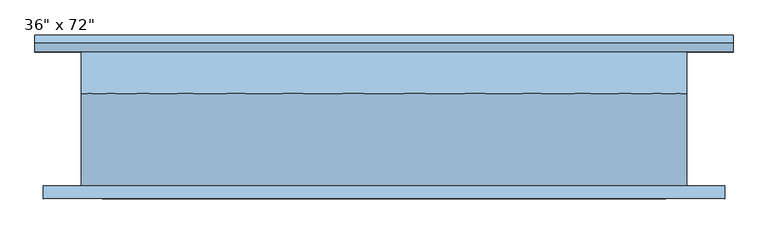
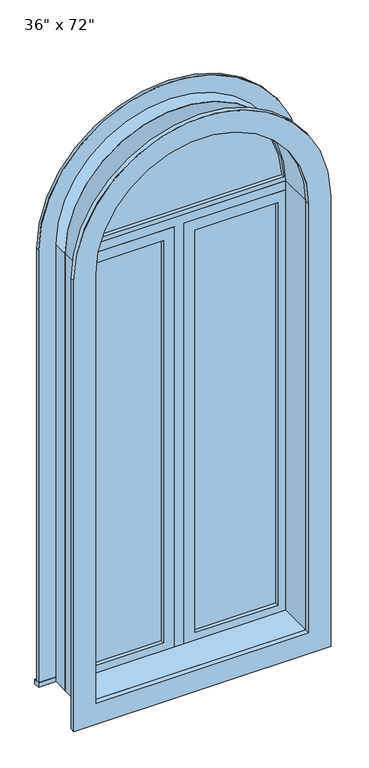
"""IFC4 building model written with IfcOpenShell, lengths in millimetres: window geometry."""

from ifc_helpers import new_model, si_unit, point, frame, frame_2d, origin, place, context, project, spatial, polyline, circle_curve, trimmed, segment, composite_curve, outline, extrude, source, transform, mapped, element, save


def window_4e95f2a8(model_context):
    return source(origin(), model_context, "Body", "SweptSolid", [
        extrude(outline(composite_curve([segment(polyline([(2152.65, -506.3478419), (247.65, -506.3478419), (247.65, 522.3521581), (2152.65, 522.3521581)]), True, "CONTINUOUS"), segment(trimmed(circle_curve(frame_2d((2152.65, 8.0021581)), 514.35), [point((2152.65, 522.3521581))], [point((2152.65, -506.3478419))], False, "CARTESIAN"), True, "CONTINUOUS")], self_intersect=False), holes=[composite_curve([segment(trimmed(circle_curve(frame_2d((2152.65, 8.0021581)), 425.45), [point((2152.65, -417.4478419))], [point((2152.65, 433.4521581))], True, "CARTESIAN"), True, "CONTINUOUS"), segment(polyline([(2152.65, 433.4521581), (336.55, 433.4521581), (336.55, -417.4478419), (2152.65, -417.4478419)]), True, "CONTINUOUS")], self_intersect=False)]), frame((0.0, -120.65, 0.0), z_axis=(0.0, 1.0, 0.0), x_axis=(0.0, 0.0, 1.0)), (0.0, 0.0, 1.0), 19.05),
        extrude(outline(composite_curve([segment(trimmed(circle_curve(frame_2d((2152.65, 8.0021581)), 419.2154707), [point((2171.6999995, 426.7845699))], [point((2171.6999995, -410.7802537))], False, "CARTESIAN"), True, "CONTINUOUS"), segment(polyline([(2171.6999995, -410.7802537), (2171.6999995, 426.7845699)]), True, "CONTINUOUS")], self_intersect=False)), frame((0.0, 53.975, 0.0), z_axis=(0.0, 1.0, 0.0), x_axis=(0.0, 0.0, 1.0)), (0.0, 0.0, 1.0), 12.7),
        extrude(outline(composite_curve([segment(trimmed(circle_curve(frame_2d((2152.65, 8.0021581)), 438.15), [point((2152.65, 446.1521581))], [point((2152.65, -430.1478419))], False, "CARTESIAN"), True, "CONTINUOUS"), segment(polyline([(2152.65, -430.1478419), (2152.65, 446.1521581)]), True, "CONTINUOUS")], self_intersect=False), holes=[composite_curve([segment(polyline([(2171.6999995, 426.7845698), (2171.6999995, -410.7802537)]), True, "CONTINUOUS"), segment(trimmed(circle_curve(frame_2d((2152.65, 8.0021581)), 419.2154707), [point((2171.6999995, -410.7802537))], [point((2171.6999995, 426.7845698))], True, "CARTESIAN"), True, "CONTINUOUS")], self_intersect=False)]), frame((0.0, 38.1, 0.0), z_axis=(0.0, 1.0, 0.0), x_axis=(0.0, 0.0, 1.0)), (0.0, 0.0, 1.0), 44.45),
        extrude(outline(composite_curve([segment(polyline([(304.8, -449.1978419), (304.8, 465.2021581), (2152.65, 465.2021581)]), True, "CONTINUOUS"), segment(trimmed(circle_curve(frame_2d((2152.65, 8.0021581)), 457.2), [point((2152.65, 465.2021581))], [point((2152.65, -449.1978419))], False, "CARTESIAN"), True, "CONTINUOUS"), segment(polyline([(2152.65, -449.1978419), (304.8, -449.1978419)]), True, "CONTINUOUS")], self_intersect=False), holes=[composite_curve([segment(polyline([(323.85, -430.1478419), (2152.65, -430.1478419)]), True, "CONTINUOUS"), segment(trimmed(circle_curve(frame_2d((2152.65, 8.0021581)), 438.15), [point((2152.65, -430.1478419))], [point((2152.65, 446.1521581))], True, "CARTESIAN"), True, "CONTINUOUS"), segment(polyline([(2152.65, 446.1521581), (323.85, 446.1521581), (323.85, -430.1478419)]), True, "CONTINUOUS")], self_intersect=False)]), frame((0.0, 38.1, 0.0), z_axis=(0.0, 1.0, 0.0), x_axis=(0.0, 0.0, 1.0)), (0.0, 0.0, 1.0), 63.5),
        extrude(outline(polyline([(71.5021581, 66.675), (401.7021581, 66.675), (401.7021581, 53.975), (71.5021581, 53.975), (71.5021581, 66.675)])), frame((0.0, 0.0, 368.3), z_axis=(0.0, 0.0, 1.0), x_axis=(1.0, 0.0, 0.0)), (0.0, 0.0, 1.0), 1701.8),
        extrude(outline(polyline([(2114.55, 27.0521581), (323.85, 27.0521581), (323.85, 446.1521581), (2114.55, 446.1521581), (2114.55, 27.0521581)]), holes=[polyline([(2070.1, 71.5021581), (2070.1, 401.7021581), (368.3, 401.7021581), (368.3, 71.5021581), (2070.1, 71.5021581)])]), frame((0.0, 38.1, 0.0), z_axis=(0.0, 1.0, 0.0), x_axis=(0.0, 0.0, 1.0)), (0.0, 0.0, 1.0), 44.45),
        extrude(outline(polyline([(323.85, -11.0478419), (323.85, 27.0521581), (2114.55, 27.0521581), (2114.55, 446.1521581), (2152.65, 446.1521581), (2152.65, -430.1478419), (2114.55, -430.1478419), (2114.55, -11.0478419), (323.85, -11.0478419)])), frame((0.0, 38.1, 0.0), z_axis=(0.0, 1.0, 0.0), x_axis=(0.0, 0.0, 1.0)), (0.0, 0.0, 1.0), 63.5),
        extrude(outline(polyline([(-519.0478419, 127.0), (535.0521581, 127.0), (535.0521581, 101.6), (-519.0478419, 101.6), (-519.0478419, 127.0)])), frame((0.0, 0.0, 304.8), z_axis=(0.0, 0.0, 1.0), x_axis=(1.0, 0.0, 0.0)), (0.0, 0.0, 1.0), 19.05),
        extrude(outline(composite_curve([segment(polyline([(323.85, 446.1521581), (323.85, 535.0521581), (2152.65, 535.0521581)]), True, "CONTINUOUS"), segment(trimmed(circle_curve(frame_2d((2152.65, 8.0021581)), 527.05), [point((2152.65, 535.0521581))], [point((2152.65, -519.0478419))], False, "CARTESIAN"), True, "CONTINUOUS"), segment(polyline([(2152.65, -519.0478419), (323.85, -519.0478419), (323.85, -430.1478419), (2152.65, -430.1478419)]), True, "CONTINUOUS"), segment(trimmed(circle_curve(frame_2d((2152.65, 8.0021581)), 438.15), [point((2152.65, -430.1478419))], [point((2152.65, 446.1521581))], True, "CARTESIAN"), True, "CONTINUOUS"), segment(polyline([(2152.65, 446.1521581), (323.85, 446.1521581)]), True, "CONTINUOUS")], self_intersect=False)), frame((0.0, 101.6, 0.0), z_axis=(0.0, 1.0, 0.0), x_axis=(0.0, 0.0, 1.0)), (0.0, 0.0, 1.0), 12.7),
        extrude(outline(polyline([(-55.4978419, 53.975), (-385.6978419, 53.975), (-385.6978419, 66.675), (-55.4978419, 66.675), (-55.4978419, 53.975)])), frame((0.0, 0.0, 368.3), z_axis=(0.0, 0.0, 1.0), x_axis=(1.0, 0.0, 0.0)), (0.0, 0.0, 1.0), 1701.8),
        extrude(outline(polyline([(2114.55, -430.1478419), (323.85, -430.1478419), (323.85, -11.0478419), (2114.55, -11.0478419), (2114.55, -430.1478419)]), holes=[polyline([(2070.1, -385.6978419), (2070.1, -55.4978419), (368.3, -55.4978419), (368.3, -385.6978419), (2070.1, -385.6978419)])]), frame((0.0, 38.1, 0.0), z_axis=(0.0, 1.0, 0.0), x_axis=(0.0, 0.0, 1.0)), (0.0, 0.0, 1.0), 44.45),
        extrude(outline(composite_curve([segment(polyline([(304.8, 465.2021581), (2152.65, 465.2021581)]), True, "CONTINUOUS"), segment(trimmed(circle_curve(frame_2d((2152.65, 8.0021581)), 457.2), [point((2152.65, 465.2021581))], [point((2152.65, -449.1978419))], False, "CARTESIAN"), True, "CONTINUOUS"), segment(polyline([(2152.65, -449.1978419), (304.8, -449.1978419), (304.8, 465.2021581)]), True, "CONTINUOUS")], self_intersect=False), holes=[composite_curve([segment(polyline([(336.55, 433.4521581), (336.55, -417.4478419), (2152.65, -417.4478419)]), True, "CONTINUOUS"), segment(trimmed(circle_curve(frame_2d((2152.65, 8.0021581)), 425.45), [point((2152.65, -417.4478419))], [point((2152.65, 433.4521581))], True, "CARTESIAN"), True, "CONTINUOUS"), segment(polyline([(2152.65, 433.4521581), (336.55, 433.4521581)]), True, "CONTINUOUS")], self_intersect=False)]), frame((0.0, -101.6, 0.0), z_axis=(0.0, 1.0, 0.0), x_axis=(0.0, 0.0, 1.0)), (0.0, 0.0, 1.0), 139.7),
    ])


if __name__ == "__main__":
    model = new_model("IFC4")
    model_context = context("Model", 3, world=origin())
    ifc_project = project(units=[si_unit("LENGTHUNIT", "METRE", prefix="MILLI")], contexts=[model_context])
    site = spatial("IfcSite", under=ifc_project)
    building = spatial("IfcBuilding", under=site)
    placement = place(None, origin())
    window_shape = window_4e95f2a8(model_context)
    element("IfcWindow", 1, ObjectType="36\" x 72\"", at=placement, inside=building, context=model_context, shape_type="MappedRepresentation", body=[
        mapped(window_shape, transform((0.0, 0.0, 0.0), x_axis=(1.0, 0.0, 0.0), y_axis=(0.0, 1.0, 0.0), z_axis=(0.0, 0.0, 1.0))),
    ])
    save(model, "model.ifc")

# Revit data of these elements
# Type "36\" x 72\""
#   Type Mark = "10"
#   Construction Type Id = "SGL"
#   Assembly Code = "B2020100"
#   Analytic Construction = "Large single-glazed windows"
#   Visual Light Transmittance = 0.9
#   Solar Heat Gain Coefficient = 0.86
#   Heat Transfer Coefficient (U) = 0.979472 BTU/(h·ft²·°F)
#   Height = 6' - 0"
#   Default Sill Height = 1' - 0"
#   Trim Projection - Ext. = 0' - 0 1/2"
#   Trim Projection - Int. = 0' - 0 3/4"
#   Trim Width - Exterior = 0' - 3 1/2"
#   Trim Width - Interior = 0' - 3 1/2"
#   Width = 3' - 0"
#   Window Inset = 0' - 0 3/4"
#   Define Thermal Properties by = 1
#   Glass Pane Material = Glass
#   Sash Material = Sash
#   Trim Exterior Material = Trim
#   Trim Interior Material = Trim
#   Wall Closure = (empty or 0)
# Element 1 (IfcWindow, "36\" x 72\"")
#   Materials on its faces: "Sash", "Trim", "Glass"
# Materials
#   "Glass": class "Glass", colour RGB 0 128 192, transparency 0.75, Description = "Soda Lime Glass", Cost = 0
#   "Sash": class "Wood", colour RGB 224 178 126, transparency 0
#   "Trim": class "Wood", colour RGB 224 178 126, transparency 0
